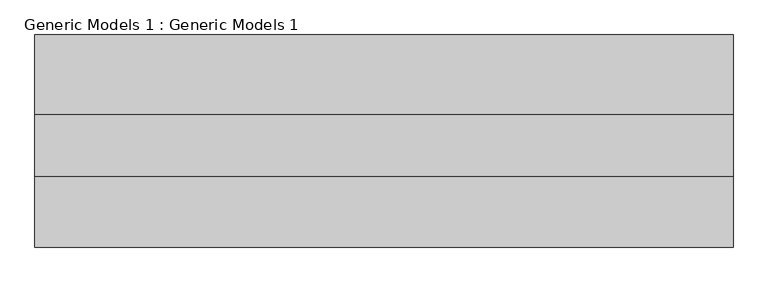
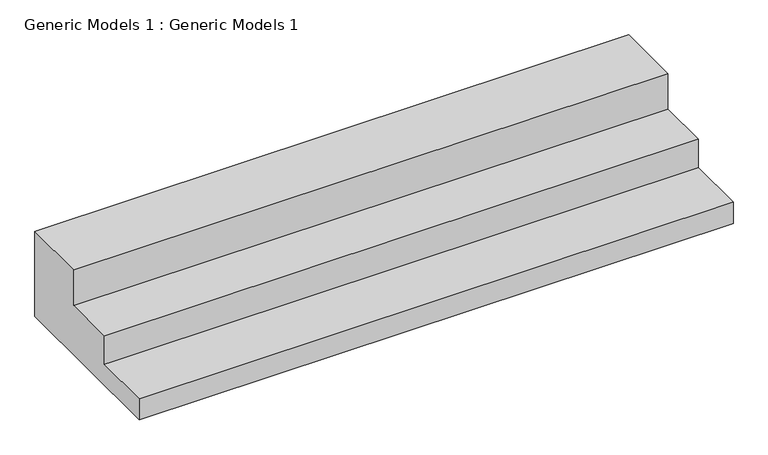
"""IFC4 building model written with IfcOpenShell, lengths in millimetres: proxy geometry, Generic Models 1 : Generic Models 1."""

from ifc_helpers import new_model, si_unit, frame, origin, place, context, project, spatial, polyline, outline, extrude, source, transform, mapped, element, save


def generic_models_1_generic_models_1_803bd6b9(model_context):
    return source(origin(), model_context, "Body", "SweptSolid", [
        extrude(outline(polyline([(-1840.2776789, 0.0), (-2449.8776789, 0.0), (-2449.8776789, 76.2), (-2246.6776789, 76.2), (-2246.6776789, 177.8), (-2068.8776789, 177.8), (-2068.8776789, 304.8), (-1840.2776789, 304.8), (-1840.2776789, 0.0)])), frame((-662.4328791, 0.0, 0.0), z_axis=(1.0, 0.0, 0.0), x_axis=(0.0, 1.0, 0.0)), (0.0, 0.0, 1.0), 2006.6),
    ])


if __name__ == "__main__":
    model = new_model("IFC4")
    model_context = context("Model", 3, world=origin())
    ifc_project = project(units=[si_unit("LENGTHUNIT", "METRE", prefix="MILLI")], contexts=[model_context])
    site = spatial("IfcSite", under=ifc_project)
    building = spatial("IfcBuilding", under=site)
    placement = place(None, origin())
    generic_models_1_generic_models_1_shape = generic_models_1_generic_models_1_803bd6b9(model_context)
    element("IfcBuildingElementProxy", 1, Name="Generic Models 1 : Generic Models 1", ObjectType="Generic Models 1 : Generic Models 1", at=placement, inside=building, context=model_context, shape_type="MappedRepresentation", body=[
        mapped(generic_models_1_generic_models_1_shape, transform((0.0, 0.0, 0.0), x_axis=(1.0, 0.0, 0.0), y_axis=(0.0, 1.0, 0.0), z_axis=(0.0, 0.0, 1.0))),
    ])
    save(model, "model.ifc")

# Revit data of these elements
# Element 1 (IfcBuildingElementProxy, "Generic Models 1 : Generic Models 1")
#   Materials on its faces: "Clad - White"
# Materials
#   "Clad - White": class "Wood", colour RGB 242 242 238, transparency 0, Cost = 0
